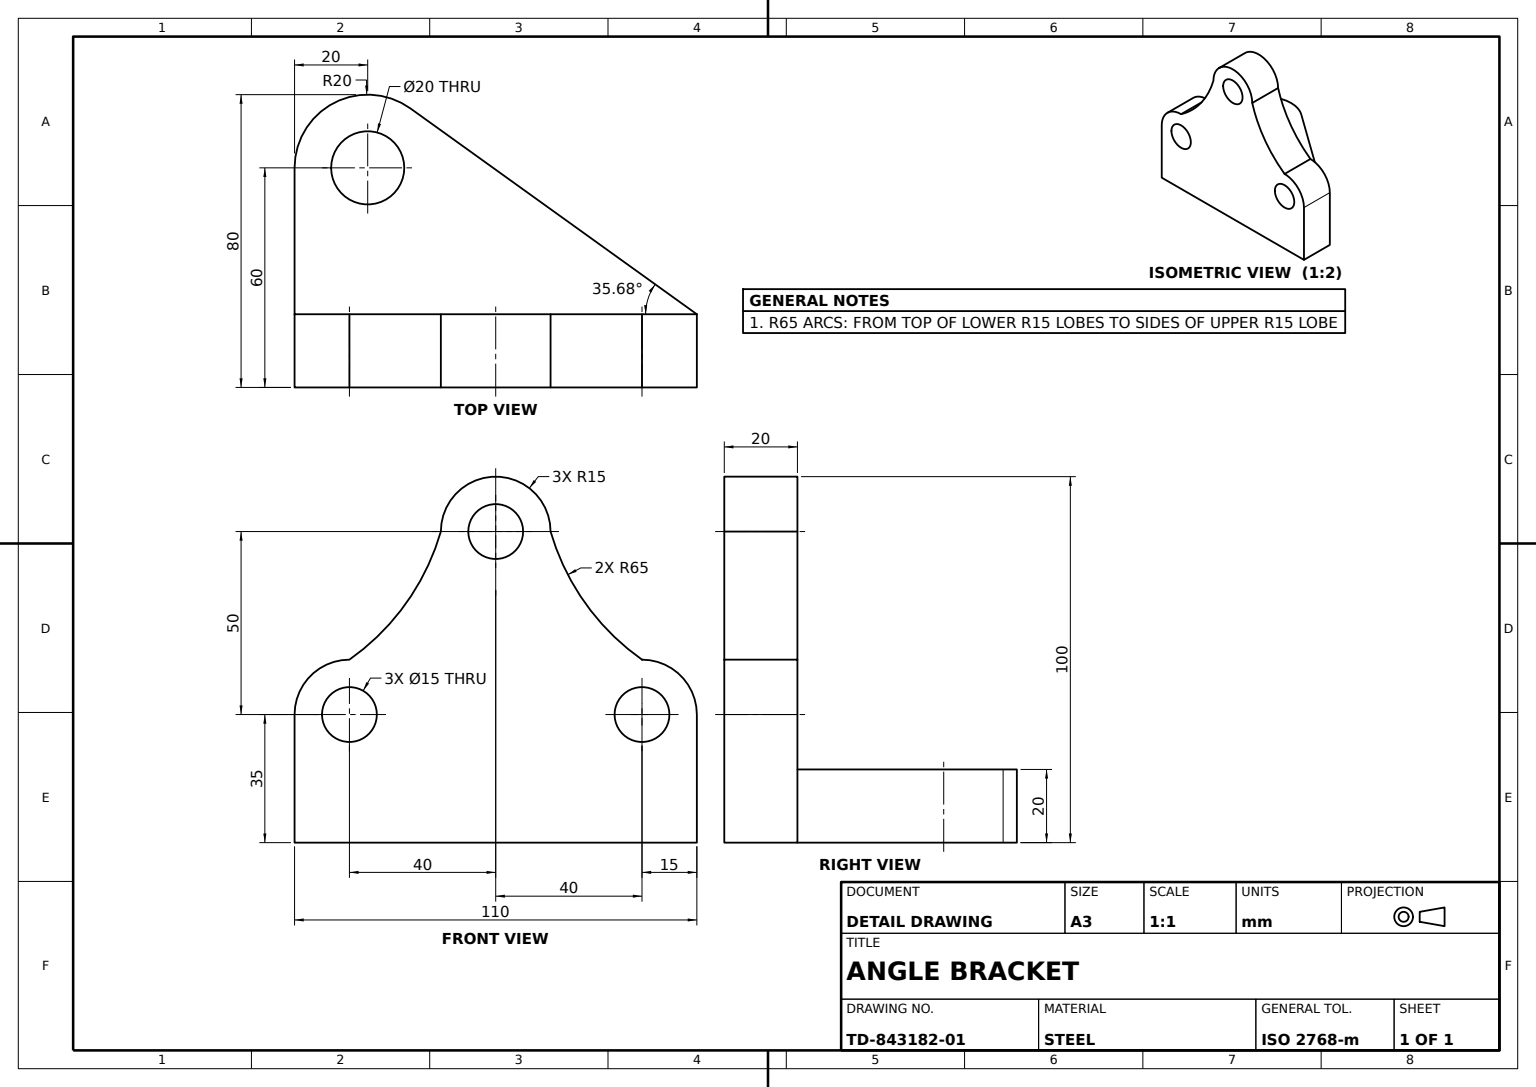
from build123d import *

# Parameters (mm, degrees)
BRACKET_PROFILE_SKETCH_R   = 7.5
BRACKET_PROFILE_BOSS_DEPTH = 20
BASE_BLOCK_SKETCH_R        = 10
BASE_BLOCK_BOSS_DEPTH      = 20


with BuildPart() as part:
    # Bracket Profile Sketch → Bracket Profile Boss (new body)
    with BuildSketch(Plane(origin=(0, 0, 0), x_dir=(0, 0, -1), z_dir=(1, 0, 0))):
        with BuildLine():
            Line((55, 0), (55, -15))
            Line((55, -15), (-55.001498604, -15))
            Line((-55.001498604, -15), (-55, 0))
            ThreePointArc((-55, 0), (-50.606601718, 10.606601718), (-40, 15))
            ThreePointArc((-40, 15), (-24.521101379, 30.372215271), (-15, 50))
            ThreePointArc((-15, 50), (0, 65), (15, 50))
            ThreePointArc((15, 50), (24.521101379, 30.372215271), (40, 15))
            ThreePointArc((40, 15), (50.606601718, 10.606601718), (55, 0))
        make_face()
        with Locations((0, 50)):
            Circle(BRACKET_PROFILE_SKETCH_R, mode=Mode.SUBTRACT)
        with Locations((40, 0)):
            Circle(BRACKET_PROFILE_SKETCH_R, mode=Mode.SUBTRACT)
        with Locations((-40, 0)):
            Circle(BRACKET_PROFILE_SKETCH_R, mode=Mode.SUBTRACT)
    extrude(amount=BRACKET_PROFILE_BOSS_DEPTH)

    # Base Block Sketch → Base Block Boss (add)
    with BuildSketch(Plane(origin=(0, -15, 0), x_dir=(-1, 0, 0), z_dir=(0, -1, 0))):
        with BuildLine():
            Line((-20, 55), (-20, -55.001498604))
            Line((-20, -55.001498604), (0, -55.001498604))
            Line((0, -55.001498604), (40, -55.001498604))
            ThreePointArc((40, -55.001498604), (57.794589541, -44.131262187), (56.246039556, -23.336756912))
            Line((56.246039556, -23.336756912), (0, 55))
            Line((0, 55), (-20, 55))
        make_face()
        with Locations(Location((40, -35.001498604, 0), (0, 0, 90))):
            Circle(BASE_BLOCK_SKETCH_R, mode=Mode.SUBTRACT)
    extrude(amount=BASE_BLOCK_BOSS_DEPTH)


solid = part.part
